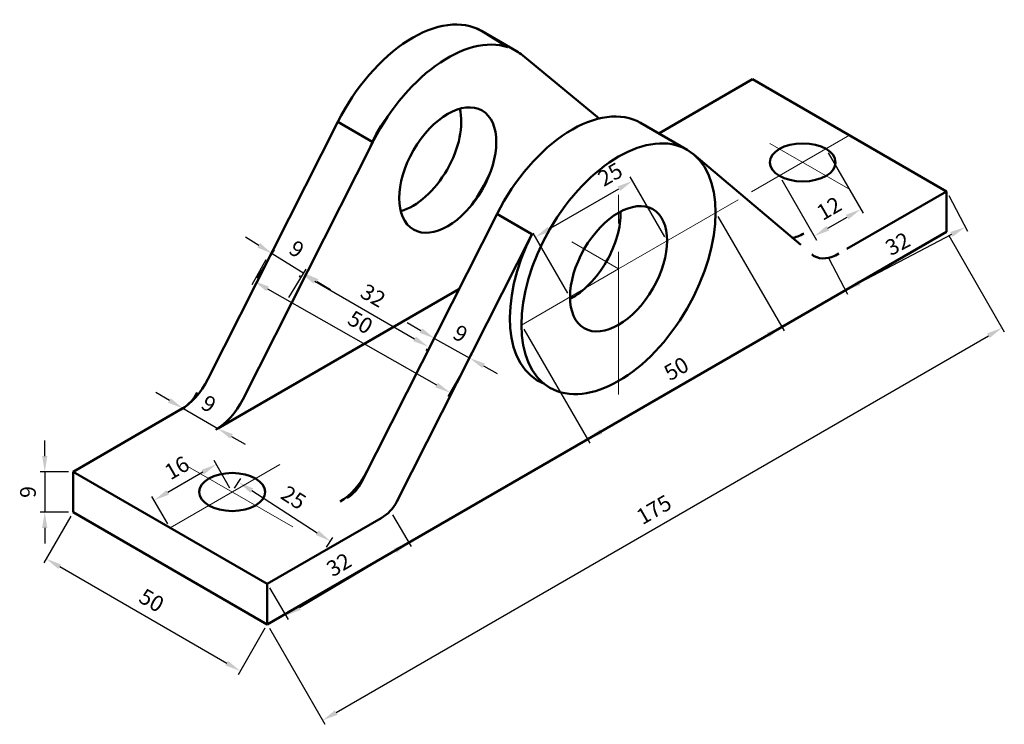
# Model space of a CAD drawing. Units: millimetres. Extents: x 2756 to 2976, y 762 to 920.
import ezdxf

# ---------------------------------------------------------------- set-up
doc = ezdxf.new("R2010")
doc.units = ezdxf.units.MM
doc.linetypes.add('CENTER', pattern=[50.8, 31.75, -6.35, 6.35, -6.35])
for name, color, linetype, lineweight in [('M-CNTR', 4, 'CENTER', 18), ('M-DIMS', 3, 'Continuous', 25), ('M-OUTL', 7, 'Continuous', 50)]:
    doc.layers.add(name, color=color, linetype=linetype, lineweight=lineweight)
doc.styles.get("Standard").update_dxf_attribs({"font": 'arial.ttf'})
doc.dimstyles.new('AM_ISO$0', dxfattribs={"dimtxt": 3.5, "dimasz": 3.5, "dimexe": 1, "dimexo": 1, "dimgap": 1.5, "dimtad": 1, "dimdsep": 46, "dimtxsty": 'Standard', "dimcen": 0, "dimclrd": 256, "dimclre": 256, "dimclrt": 2, "dimadec": 0, "dimazin": 2, "dimtp": 0.1, "dimtm": 0.1, "dimtfac": 0.71, "dimtdec": 3, "dimtmove": 0, "dimatfit": 3, "dimfxl": 1, "dimlwd": -1, "dimlwe": -1, "dimarcsym": 1})

# ---------------------------------------------------------------- blocks, each defined once
blk = doc.blocks.new('*D3')
at = {"layer": 'Defpoints', "color": 0, "transparency": 16777216}
for p in [(2962.88, 872.26), (2975.24, 850.85), (2811.33, 784.76)]:
    blk.add_point(p, dxfattribs=at)
at = {"layer": 'M-DIMS', "color": 0, "linetype": 'ByBlock', "transparency": 16777216}
for p, q in [((2963.38, 871.4), (2975.74, 849.99)), ((2826.72, 765.1), (2972.21, 849.1)), ((2811.83, 783.9), (2824.18, 762.49))]:
    blk.add_line(p, q, dxfattribs=at)
at = {"layer": 'M-DIMS', "color": 0, "transparency": 16777216}
for points in [[(2971.92, 849.61), (2972.5, 848.6), (2975.24, 850.85)], [(2826.42, 765.61), (2827.01, 764.6), (2823.68, 763.35)]]:
    blk.add_solid(points, dxfattribs=at)
at = {"layer": 'M-DIMS', "color": 0, "transparency": 16777216, "insert": (2897.82, 809.95), "char_height": 3.5, "attachment_point": 5, "rotation": 30}
blk.add_mtext('175', dxfattribs=at)
blk = doc.blocks.new('*D4')
at = {"layer": 'Defpoints', "color": 0, "transparency": 16777216}
for p in [(2962.88, 881.26), (2936.14, 867.22), (2940.32, 859.26)]:
    blk.add_point(p, dxfattribs=at)
at = {"layer": 'M-DIMS', "color": 0, "linetype": 'ByBlock', "transparency": 16777216}
for p, q in [((2963.34, 880.38), (2967.52, 872.42)), ((2963.96, 871.68), (2943.42, 860.89)), ((2936.61, 866.33), (2940.79, 858.38))]:
    blk.add_line(p, q, dxfattribs=at)
at = {"layer": 'M-DIMS', "color": 0, "transparency": 16777216}
for points in [[(2963.69, 872.19), (2964.23, 871.16), (2967.06, 873.3)], [(2943.15, 861.41), (2943.69, 860.37), (2940.32, 859.26)]]:
    blk.add_solid(points, dxfattribs=at)
at = {"layer": 'M-DIMS', "color": 0, "transparency": 16777216, "insert": (2952.16, 869.19), "char_height": 3.5, "attachment_point": 5, "rotation": 27.7118}
blk.add_mtext('32', dxfattribs=at)
blk = doc.blocks.new('*D5')
at = {"layer": 'Defpoints', "color": 0, "transparency": 16777216}
for p in [(2838.75, 810.03), (2842.93, 802.99), (2811.33, 793.76)]:
    blk.add_point(p, dxfattribs=at)
at = {"layer": 'M-DIMS', "color": 0, "linetype": 'ByBlock', "transparency": 16777216}
for p, q in [((2839.26, 809.17), (2843.44, 802.13)), ((2818.51, 788.51), (2839.92, 801.2)), ((2811.84, 792.9), (2816.01, 785.86))]:
    blk.add_line(p, q, dxfattribs=at)
at = {"layer": 'M-DIMS', "color": 0, "transparency": 16777216}
for points in [[(2839.62, 801.71), (2840.22, 800.7), (2842.93, 802.99)], [(2818.21, 789.01), (2818.81, 788.01), (2815.5, 786.72)]]:
    blk.add_solid(points, dxfattribs=at)
at = {"layer": 'M-DIMS', "color": 0, "transparency": 16777216, "insert": (2827.54, 797.68), "char_height": 3.5, "attachment_point": 5, "rotation": 30.6728}
blk.add_mtext('32', dxfattribs=at)
blk = doc.blocks.new('*D6')
at = {"layer": 'Defpoints', "color": 0, "transparency": 16777216}
for p in [(2792.53, 832.91), (2800.32, 828.41), (2800.32, 828.41)]:
    blk.add_point(p, dxfattribs=at)
at = {"layer": 'M-DIMS', "color": 0, "linetype": 'ByBlock', "transparency": 16777216}
for p, q in [((2789.5, 834.66), (2786.47, 836.41)), ((2792.53, 832.91), (2800.32, 828.41)), ((2803.35, 826.66), (2806.39, 824.91))]:
    blk.add_line(p, q, dxfattribs=at)
at = {"layer": 'M-DIMS', "color": 0, "transparency": 16777216}
for points in [[(2789.79, 835.17), (2789.21, 834.16), (2792.53, 832.91)], [(2803.65, 827.17), (2803.06, 826.16), (2800.32, 828.41)]]:
    blk.add_solid(points, dxfattribs=at)
at = {"layer": 'M-DIMS', "color": 0, "transparency": 16777216, "insert": (2798.07, 833.51), "char_height": 3.5, "attachment_point": 5, "rotation": 330}
blk.add_mtext('9', dxfattribs=at)
blk = doc.blocks.new('*D7')
at = {"layer": 'Defpoints', "color": 0, "transparency": 16777216}
for p in [(2768.02, 818.76), (2761.71, 809.76), (2768.02, 809.76)]:
    blk.add_point(p, dxfattribs=at)
at = {"layer": 'M-DIMS', "color": 0, "linetype": 'ByBlock', "transparency": 16777216}
for p, q in [((2761.71, 822.26), (2761.71, 825.76)), ((2767.02, 818.76), (2760.71, 818.76)), ((2761.71, 818.76), (2761.71, 809.76)), ((2767.02, 809.76), (2760.71, 809.76)), ((2761.71, 806.26), (2761.71, 802.76))]:
    blk.add_line(p, q, dxfattribs=at)
at = {"layer": 'M-DIMS', "color": 0, "transparency": 16777216}
for points in [[(2761.12, 822.26), (2762.29, 822.26), (2761.71, 818.76)], [(2761.12, 806.26), (2762.29, 806.26), (2761.71, 809.76)]]:
    blk.add_solid(points, dxfattribs=at)
at = {"layer": 'M-DIMS', "color": 0, "transparency": 16777216, "insert": (2758.42, 814.26), "char_height": 3.5, "attachment_point": 5, "rotation": 90}
blk.add_mtext('9', dxfattribs=at)
blk = doc.blocks.new('*D8')
at = {"layer": 'Defpoints', "color": 0, "transparency": 16777216}
for p in [(2768.02, 809.76), (2811.33, 784.76), (2805.33, 774.37)]:
    blk.add_point(p, dxfattribs=at)
at = {"layer": 'M-DIMS', "color": 0, "linetype": 'ByBlock', "transparency": 16777216}
for p, q in [((2767.52, 808.9), (2761.52, 798.5)), ((2765.06, 797.62), (2802.29, 776.12)), ((2810.83, 783.9), (2804.83, 773.5))]:
    blk.add_line(p, q, dxfattribs=at)
at = {"layer": 'M-DIMS', "color": 0, "transparency": 16777216}
for points in [[(2765.35, 798.12), (2764.76, 797.11), (2762.02, 799.37)], [(2802.59, 776.62), (2802, 775.61), (2805.33, 774.37)]]:
    blk.add_solid(points, dxfattribs=at)
at = {"layer": 'M-DIMS', "color": 0, "transparency": 16777216, "insert": (2785.32, 789.72), "char_height": 3.5, "attachment_point": 5, "rotation": 330}
blk.add_mtext('50', dxfattribs=at)
blk = doc.blocks.new('*D9')
at = {"layer": 'Defpoints', "color": 0, "transparency": 16777216}
for p in [(2803.53, 814.26), (2786.12, 812.43), (2789.67, 806.26)]:
    blk.add_point(p, dxfattribs=at)
at = {"layer": 'M-DIMS', "color": 0, "linetype": 'ByBlock', "transparency": 16777216}
for p, q in [((2803.03, 815.13), (2799.47, 821.29)), ((2796.94, 818.68), (2789.15, 814.18)), ((2789.17, 807.13), (2785.62, 813.29))]:
    blk.add_line(p, q, dxfattribs=at)
at = {"layer": 'M-DIMS', "color": 0, "transparency": 16777216}
for points in [[(2796.65, 819.18), (2797.23, 818.17), (2799.97, 820.43)], [(2788.86, 814.68), (2789.44, 813.67), (2786.12, 812.43)]]:
    blk.add_solid(points, dxfattribs=at)
at = {"layer": 'M-DIMS', "color": 0, "transparency": 16777216, "insert": (2791.4, 819.27), "char_height": 3.5, "attachment_point": 5, "rotation": 30}
blk.add_mtext('16', dxfattribs=at)
blk = doc.blocks.new('*D10')
at = {"layer": 'Defpoints', "color": 0, "transparency": 16777216}
for p in [(2803.53, 814.26), (2825.43, 803.29), (2824.02, 801.09)]:
    blk.add_point(p, dxfattribs=at)
at = {"layer": 'M-DIMS', "color": 0, "linetype": 'ByBlock', "transparency": 16777216}
for p, q in [((2804.07, 815.1), (2805.48, 817.3)), ((2807.89, 814.57), (2822.49, 805.18)), ((2824.56, 801.93), (2825.97, 804.13))]:
    blk.add_line(p, q, dxfattribs=at)
at = {"layer": 'M-DIMS', "color": 0, "transparency": 16777216}
for points in [[(2808.2, 815.06), (2807.57, 814.08), (2804.94, 816.46)], [(2822.8, 805.67), (2822.17, 804.69), (2825.43, 803.29)]]:
    blk.add_solid(points, dxfattribs=at)
at = {"layer": 'M-DIMS', "color": 0, "transparency": 16777216, "insert": (2816.97, 812.64), "char_height": 3.5, "attachment_point": 5, "rotation": 327.2685}
blk.add_mtext('25', dxfattribs=at)
blk = doc.blocks.new('*D11')
at = {"layer": 'Defpoints', "color": 0, "transparency": 16777216}
for p in [(2911.35, 876.51), (2868.05, 851.43), (2926.1, 851.05)]:
    blk.add_point(p, dxfattribs=at)
at = {"layer": 'M-DIMS', "color": 0, "linetype": 'ByBlock', "transparency": 16777216}
for p, q in [((2911.85, 875.65), (2926.6, 850.19)), ((2868.55, 850.57), (2883.3, 825.11)), ((2885.82, 827.73), (2923.07, 849.3))]:
    blk.add_line(p, q, dxfattribs=at)
at = {"layer": 'M-DIMS', "color": 0, "transparency": 16777216}
for points in [[(2922.78, 849.8), (2923.36, 848.79), (2926.1, 851.05)], [(2885.53, 828.23), (2886.12, 827.22), (2882.8, 825.97)]]:
    blk.add_solid(points, dxfattribs=at)
at = {"layer": 'M-DIMS', "color": 0, "transparency": 16777216, "insert": (2902.8, 841.36), "char_height": 3.5, "attachment_point": 5, "rotation": 30.0776}
blk.add_mtext('50', dxfattribs=at)
blk = doc.blocks.new('*D12')
at = {"layer": 'Defpoints', "color": 0, "transparency": 16777216}
for p in [(2892.8, 883.61), (2900.53, 870.26), (2878.88, 857.72)]:
    blk.add_point(p, dxfattribs=at)
at = {"layer": 'M-DIMS', "color": 0, "linetype": 'ByBlock', "transparency": 16777216}
for p, q in [((2900.02, 871.13), (2892.3, 884.47)), ((2874.17, 872.82), (2889.77, 881.85)), ((2878.37, 858.59), (2870.64, 871.93))]:
    blk.add_line(p, q, dxfattribs=at)
at = {"layer": 'M-DIMS', "color": 0, "transparency": 16777216}
for points in [[(2889.48, 882.36), (2890.06, 881.35), (2892.8, 883.61)], [(2873.88, 873.33), (2874.47, 872.32), (2871.15, 871.07)]]:
    blk.add_solid(points, dxfattribs=at)
at = {"layer": 'M-DIMS', "color": 0, "transparency": 16777216, "insert": (2888.05, 884.66), "char_height": 3.5, "attachment_point": 5, "rotation": 30.0776}
blk.add_mtext('25', dxfattribs=at)
blk = doc.blocks.new('*D13')
at = {"layer": 'Defpoints', "color": 0, "transparency": 16777216}
for p in [(2811.54, 866.87), (2855.32, 841.97), (2852.15, 836.38)]:
    blk.add_point(p, dxfattribs=at)
at = {"layer": 'M-DIMS', "color": 0, "linetype": 'ByBlock', "transparency": 16777216}
for p, q in [((2811.05, 866), (2807.87, 860.41)), ((2811.4, 859.55), (2849.1, 838.11)), ((2854.83, 841.1), (2851.65, 835.51))]:
    blk.add_line(p, q, dxfattribs=at)
at = {"layer": 'M-DIMS', "color": 0, "transparency": 16777216}
for points in [[(2811.69, 860.06), (2811.12, 859.04), (2808.36, 861.28)], [(2849.39, 838.62), (2848.82, 837.6), (2852.15, 836.38)]]:
    blk.add_solid(points, dxfattribs=at)
at = {"layer": 'M-DIMS', "color": 0, "transparency": 16777216, "insert": (2831.88, 851.69), "char_height": 3.5, "attachment_point": 5, "rotation": 330.3692}
blk.add_mtext('50', dxfattribs=at)
blk = doc.blocks.new('*D14')
at = {"layer": 'Defpoints', "color": 0, "transparency": 16777216}
for p in [(2808.53, 861.09), (2819.48, 863.04), (2815.59, 856.73)]:
    blk.add_point(p, dxfattribs=at)
at = {"layer": 'M-DIMS', "color": 0, "linetype": 'ByBlock', "transparency": 16777216}
for p, q in [((2809.44, 869.23), (2806.46, 871.07)), ((2809.06, 861.94), (2812.95, 868.24)), ((2812.42, 867.39), (2819.48, 863.04)), ((2816.12, 857.58), (2820.01, 863.89)), ((2822.46, 861.2), (2825.44, 859.36))]:
    blk.add_line(p, q, dxfattribs=at)
at = {"layer": 'M-DIMS', "color": 0, "transparency": 16777216}
for points in [[(2809.75, 869.73), (2809.14, 868.73), (2812.42, 867.39)], [(2822.77, 861.7), (2822.15, 860.71), (2819.48, 863.04)]]:
    blk.add_solid(points, dxfattribs=at)
at = {"layer": 'M-DIMS', "color": 0, "transparency": 16777216, "insert": (2817.68, 868.01), "char_height": 3.5, "attachment_point": 5, "rotation": 328.3372}
blk.add_mtext('9', dxfattribs=at)
blk = doc.blocks.new('*D15')
at = {"layer": 'Defpoints', "color": 0, "transparency": 16777216}
for p in [(2819.18, 863.4), (2847.24, 846.64), (2847.48, 847.06)]:
    blk.add_point(p, dxfattribs=at)
at = {"layer": 'M-DIMS', "color": 0, "linetype": 'ByBlock', "transparency": 16777216}
for p, q in [((2818.68, 862.53), (2818.44, 862.11)), ((2821.97, 861.23), (2844.21, 848.39)), ((2846.98, 846.19), (2846.74, 845.78))]:
    blk.add_line(p, q, dxfattribs=at)
at = {"layer": 'M-DIMS', "color": 0, "transparency": 16777216}
for points in [[(2822.27, 861.73), (2821.68, 860.72), (2818.94, 862.98)], [(2844.5, 848.9), (2843.92, 847.89), (2847.24, 846.64)]]:
    blk.add_solid(points, dxfattribs=at)
at = {"layer": 'M-DIMS', "color": 0, "transparency": 16777216, "insert": (2834.73, 857.66), "char_height": 3.5, "attachment_point": 5, "rotation": 330}
blk.add_mtext('32', dxfattribs=at)
blk = doc.blocks.new('*D16')
at = {"layer": 'Defpoints', "color": 0, "transparency": 16777216}
for p in [(2847.48, 846.37), (2856.52, 844.1), (2855.32, 841.97)]:
    blk.add_point(p, dxfattribs=at)
at = {"layer": 'M-DIMS', "color": 0, "linetype": 'ByBlock', "transparency": 16777216}
for p, q in [((2845.63, 850.21), (2842.57, 851.93)), ((2847.97, 847.24), (2849.17, 849.37)), ((2848.68, 848.5), (2856.52, 844.1)), ((2855.81, 842.84), (2857.01, 844.97)), ((2859.58, 842.39), (2862.63, 840.68))]:
    blk.add_line(p, q, dxfattribs=at)
at = {"layer": 'M-DIMS', "color": 0, "transparency": 16777216}
for points in [[(2845.91, 850.72), (2845.34, 849.71), (2848.68, 848.5)], [(2859.86, 842.9), (2859.29, 841.88), (2856.52, 844.1)]]:
    blk.add_solid(points, dxfattribs=at)
at = {"layer": 'M-DIMS', "color": 0, "transparency": 16777216, "insert": (2854.21, 849.17), "char_height": 3.5, "attachment_point": 5, "rotation": 330.7083}
blk.add_mtext('9', dxfattribs=at)
blk = doc.blocks.new('*D17')
at = {"layer": 'Defpoints', "color": 0, "transparency": 16777216}
for p in [(2935.97, 890.73), (2925.58, 884.73), (2943.73, 877.29)]:
    blk.add_point(p, dxfattribs=at)
at = {"layer": 'M-DIMS', "color": 0, "linetype": 'ByBlock', "transparency": 16777216}
for p, q in [((2936.47, 889.86), (2944.23, 876.42)), ((2926.08, 883.86), (2933.84, 870.42)), ((2936.37, 873.04), (2940.7, 875.54))]:
    blk.add_line(p, q, dxfattribs=at)
at = {"layer": 'M-DIMS', "color": 0, "transparency": 16777216}
for points in [[(2940.41, 876.04), (2940.99, 875.03), (2943.73, 877.29)], [(2936.08, 873.54), (2936.66, 872.53), (2933.34, 871.29)]]:
    blk.add_solid(points, dxfattribs=at)
at = {"layer": 'M-DIMS', "color": 0, "transparency": 16777216, "insert": (2936.87, 877.09), "char_height": 3.5, "attachment_point": 5, "rotation": 30}
blk.add_mtext('12', dxfattribs=at)

msp = doc.modelspace()

# ---------------------------------------------------------------- linework, layer by layer
at = {"layer": 'M-CNTR'}
for p, q in [((2941.229, 893.762), (2919.344, 881.126)), ((2923.426, 891.969), (2940.923, 881.867)), ((2889.701, 836.012), (2889.701, 885.831)), ((2889.701, 864.012), (2916.369, 879.409)), ((2889.701, 864.012), (2879.308, 870.012)), ((2887.103, 865.512), (2889.701, 864.012)), ((2889.701, 864.012), (2868.05, 851.434)), ((2814.174, 820.407), (2789.675, 806.262)), ((2793.139, 820.262), (2817.038, 806.464))]:
    msp.add_line(p, q, dxfattribs=at)
at = {"layer": 'M-OUTL'}
for p, q in [((2859.111, 917.029), (2864.981, 913.39)), ((2866.905, 912.529), (2859.111, 917.029)), ((2868.323, 911.541), (2885.376, 897.513)), ((2919.579, 906.262), (2898.669, 894.19)), ((2962.88, 881.262), (2919.579, 906.262)), ((2798.075, 839.386), (2827.073, 896.726)), ((2834.868, 892.226), (2827.073, 896.726)), ((2894.618, 896.529), (2905.01, 890.529)), ((2805.869, 834.886), (2834.868, 892.226)), ((2835.071, 892.864), (2835.166, 892.809)), ((2930.336, 869.344), (2906.509, 889.474)), ((2962.88, 881.262), (2940.644, 868.424)), ((2962.88, 872.262), (2962.88, 881.262)), ((2832.353, 816.456), (2862.606, 876.276)), ((2870.375, 871.726), (2862.58, 876.226)), ((2811.325, 784.762), (2962.88, 872.262)), ((2870.4, 871.776), (2840.248, 812.154)), ((2868.324, 867.67), (2868.609, 867.835)), ((2800.324, 828.41), (2854.101, 859.459)), ((2768.024, 818.762), (2792.529, 832.91)), ((2768.024, 809.762), (2768.024, 818.762)), ((2768.024, 818.762), (2811.325, 793.762)), ((2811.325, 784.762), (2768.024, 809.762)), ((2811.325, 793.762), (2836.717, 808.422)), ((2811.325, 793.762), (2789.675, 806.262)), ((2811.325, 784.762), (2811.325, 793.762))]:
    msp.add_line(p, q, dxfattribs=at)
for centre, start in [((2787.677, 840.49), 302.62188), ((2824.322, 820.517), 302.62188), ((2832.217, 816.216), 300)]:
    msp.add_arc(centre, 9, start, 333.17318, dxfattribs=at)
for centre, major_axis, start_param, end_param in [((2843.801, 890.512), (15.309, 26.517), 0, 1.6683699), ((2843.801, 890.512), (-15.309, -26.517), 3.1054246, 3.2219736), ((2851.596, 886.012), (-15.309, -26.517), 3.2605091, 4.8456942), ((2851.596, 886.012), (-15.309, -26.517), 3.044019, 3.1415927), ((2843.801, 890.512), (-7.655, -13.258), 4.4433329, 4.981445), ((2843.801, 890.512), (-7.655, -13.258), 0.5341584, 2.6074342), ((2879.308, 870.012), (-15.309, -26.517), 3.1415927, 4.808119), ((2887.103, 865.512), (-15.309, -26.517), 9.339823, 9.424778), ((2843.801, 890.512), (-15.309, -26.517), 7.7206764, 7.9872869), ((2879.308, 870.012), (-7.655, -13.258), 7.0293432, 8.6786201), ((2931.048, 880.884), (5.511, 9.546), 3.5718579, 3.9269908), ((2887.103, 865.512), (-15.309, -26.517), 4.808119, 6.3681403), ((2938.842, 876.384), (5.511, 9.546), 3.0458634, 3.1415927), ((2938.842, 876.384), (5.511, 9.546), 3.1415927, 3.9269908), ((2792.062, 841.64), (-5.511, -9.546), 0.7853982, 1.6665256), ((2799.856, 837.14), (-5.511, -9.546), 0.7853982, 1.6665256), ((2827.569, 821.14), (-5.511, -9.546), 0.7853982, 1.6665256)]:
    msp.add_ellipse(centre, major_axis=major_axis, ratio=0.5773503, start_param=start_param, end_param=end_param, dxfattribs=at)
for centre, major_axis in [((2851.596, 886.012), (-7.655, -13.258)), ((2889.701, 864.012), (-15.309, -26.517)), ((2930.774, 887.726), (-7.348, 0)), ((2889.701, 864.012), (-7.655, -13.258)), ((2803.531, 814.262), (-7.348, 0))]:
    msp.add_ellipse(centre, major_axis=major_axis, ratio=0.5773503, dxfattribs=at)

# ---------------------------------------------------------------- dimensions: what is measured, and where the dimension line sits
at = {"layer": 'M-DIMS'}
dim = msp.add_linear_dim(base=(2943.729, 877.288), p1=(2925.578, 884.726), p2=(2935.97, 890.726), angle=30, dimstyle='AM_ISO$0', override={"dimclrd": 0, "dimclre": 0, "dimclrt": 0}, dxfattribs=at)
dim.commit()
dim.dimension.update_dxf_attribs({"geometry": '*D17', "text_midpoint": (2938.499, 874.269), "dimtype": 161})
for base, p1, p2, angle, text, picture, middle in [((2892.796, 883.609), (2878.875, 857.723), (2900.526, 870.262), 30.07758, '25', '*D12', (2889.701, 881.816)), ((2819.482, 863.039), (2808.533, 861.087), (2815.593, 856.733), 328.33725, '9', '*D14', (2815.952, 865.216)), ((2856.523, 844.102), (2847.48, 846.366), (2855.324, 841.965), 330.70828, '9', '*D16', (2852.6, 846.302))]:
    dim = msp.add_linear_dim(base=base, p1=p1, p2=p2, angle=angle, text=text, dimstyle='AM_ISO$0', override={"dimpost": '', "dimclrd": 0, "dimclre": 0, "dimclrt": 0}, dxfattribs=at)
    dim.commit()
    dim.dimension.update_dxf_attribs({"geometry": picture, "text_midpoint": middle, "dimtype": 161})
for p1, p2, distance, text, picture, middle in [((2962.88, 881.262), (2936.144, 867.219), 8.989, '32', '*D4', (2952.163, 869.194)), ((2868.05, 851.434), (2911.351, 876.512), -29.422, '50', '*D11', (2902.799, 841.358)), ((2811.54, 866.869), (2855.324, 841.965), -6.428, '50', '*D13', (2831.879, 851.687)), ((2819.185, 863.396), (2847.48, 847.06), -0.483, '32', '*D15', (2834.735, 857.657)), ((2803.531, 814.262), (2824.021, 801.092), 2.612, '25', '*D10', (2816.966, 812.639)), ((2811.325, 793.762), (2838.754, 810.031), -8.185, '32', '*D5', (2827.538, 797.684))]:
    dim = msp.add_aligned_dim(p1=p1, p2=p2, distance=distance, text=text, dimstyle='AM_ISO$0', override={"dimpost": '', "dimclrd": 0, "dimclre": 0, "dimclrt": 0}, dxfattribs=at)
    dim.commit()
    dim.dimension.update_dxf_attribs({"geometry": picture, "text_midpoint": middle})
for p1, p2, distance, override, picture, middle in [((2811.325, 784.762), (2962.88, 872.262), -24.719, {"dimpost": '', "dimclrd": 0, "dimclre": 0, "dimclrt": 0}, '*D3', (2897.819, 809.952)), ((2792.529, 832.91), (2800.324, 828.41), 0, {"dimclrd": 0, "dimclre": 0, "dimclrt": 0}, '*D6', (2798.07, 833.507)), ((2768.024, 818.762), (2768.024, 809.762), -6.318, {"dimclrd": 0, "dimclre": 0, "dimclrt": 0}, '*D7', (2758.419, 814.262)), ((2803.531, 814.262), (2789.675, 806.262), -7.117, {"dimclrd": 0, "dimclre": 0, "dimclrt": 0}, '*D9', (2791.401, 819.272)), ((2768.024, 809.762), (2811.325, 784.762), -12, {"dimclrd": 0, "dimclre": 0, "dimclrt": 0}, '*D8', (2785.318, 789.716))]:
    dim = msp.add_aligned_dim(p1=p1, p2=p2, distance=distance, dimstyle='AM_ISO$0', override=override, dxfattribs=at)
    dim.commit()
    dim.dimension.update_dxf_attribs({"geometry": picture, "text_midpoint": middle})

doc.saveas('drawing.dxf')
